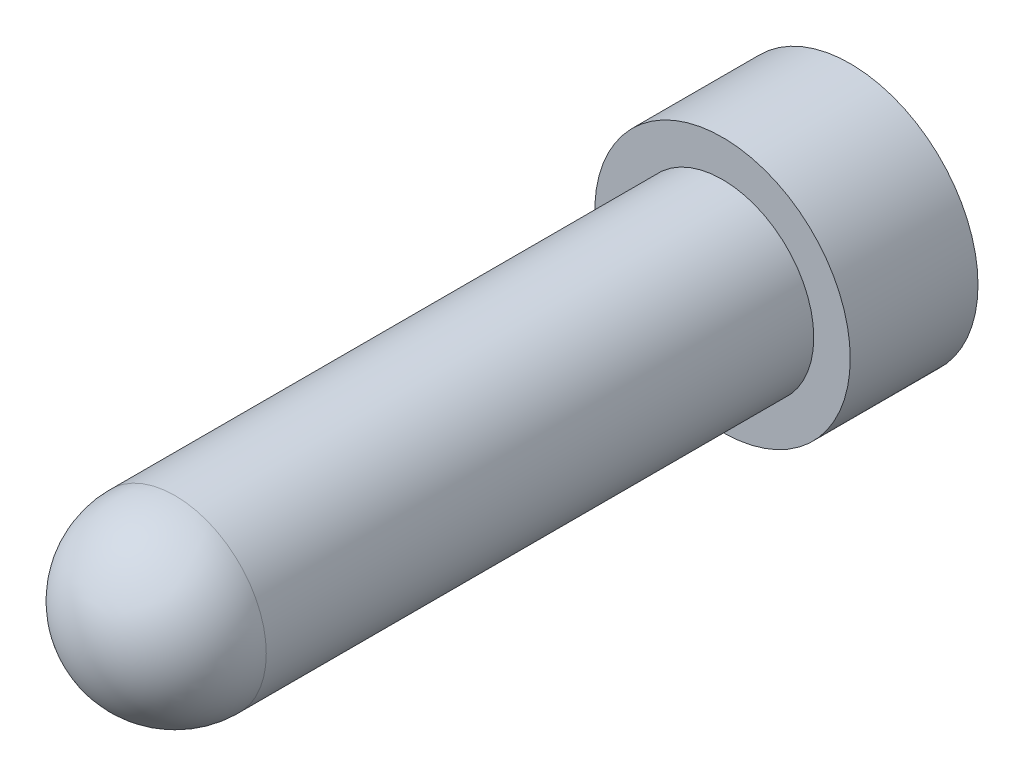
from build123d import *

# Parameters (mm, degrees)
HEAD_PROFILE_SKETCH_R       = 7
HEAD_14X10_DEPTH            = 7
SHANK_PROFILE_SKETCH_R      = 5
SHANK_10X35_DEPTH           = 35
DOMED_END_R5_R              = 5
HEX_SOCKET_CUT_5_DEEP_DEPTH = 5


with BuildPart() as part:
    # Head Profile Sketch → Head Ø14x10 (new body)
    with BuildSketch(Plane.XY):
        Circle(HEAD_PROFILE_SKETCH_R)
    extrude(amount=HEAD_14X10_DEPTH)

    # Shank Profile Sketch → Shank Ø10x35 (add)
    with BuildSketch(Plane.XY.offset(7)):
        Circle(SHANK_PROFILE_SKETCH_R)
    extrude(amount=SHANK_10X35_DEPTH)

    # Domed End R5
    domed_end_r5_edges = [part.edges().sort_by_distance(p)[0] for p in [
        (-5, 0, 42),
    ]]
    fillet(domed_end_r5_edges, radius=DOMED_END_R5_R)

    # Hex Socket Sketch → Hex Socket Cut 5 Deep (cut)
    with BuildSketch(Plane(origin=(0, 0, 0), x_dir=(-1, 0, 0), z_dir=(0, 0, -1))):
        Polygon((5.773502692, 0), (2.886751346, 5), (-2.886751346, 5), (-5.773502692, 0), (-2.886751346, -5), (2.886751346, -5), align=None)
    extrude(amount=-HEX_SOCKET_CUT_5_DEEP_DEPTH, mode=Mode.SUBTRACT)


solid = part.part
